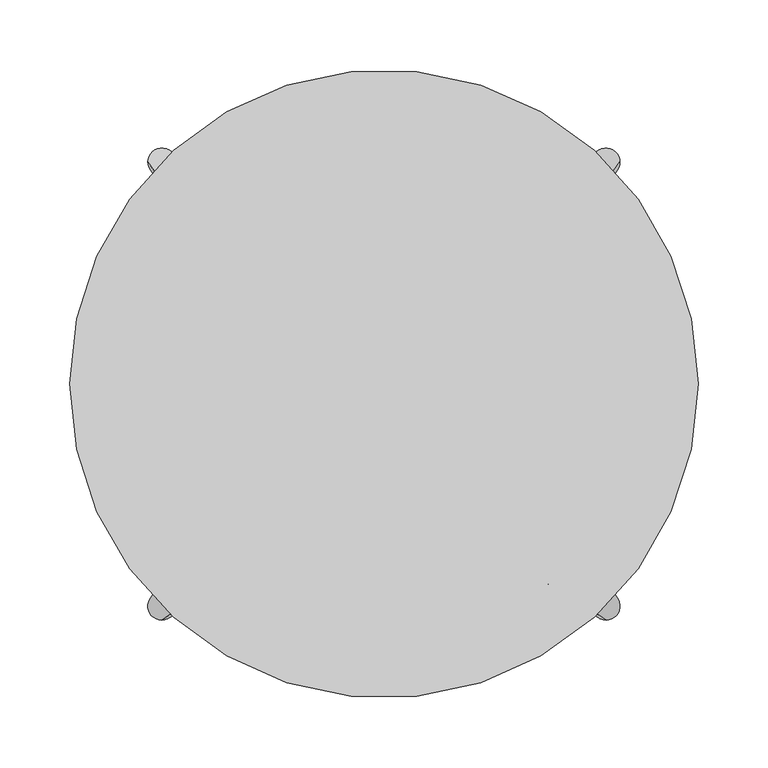
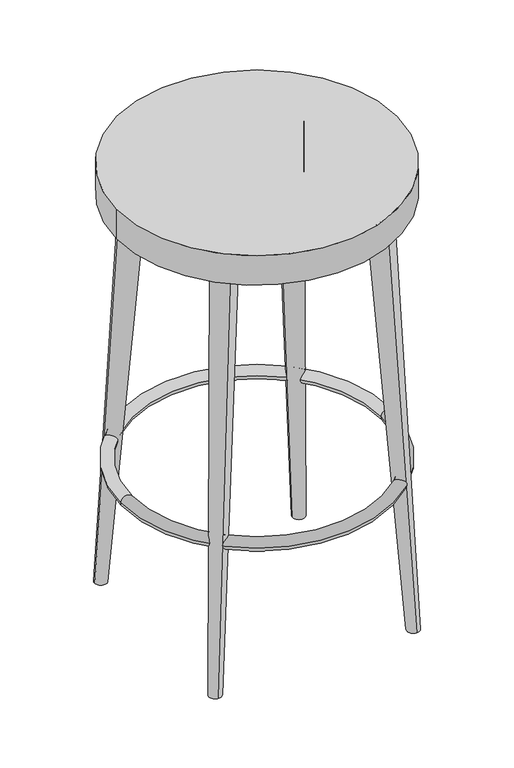
"""IFC4 building model written with IfcOpenShell, lengths in millimetres: furniture geometry."""

from ifc_helpers import new_model, si_unit, point, frame, origin, origin_2d, place, context, project, spatial, circle_curve, ellipse_curve, trimmed, segment, composite_curve, outline, extrude, source, transform, mapped, element, save
from ifc_brep_helpers import plane_surface, revolved_surface, spline_surface, advanced_brep


def furniture_d95c0d1d(model_context):
    return source(origin(), model_context, "Body", "SolidModel", [
        extrude(outline(composite_curve([segment(trimmed(circle_curve(origin_2d(), 225.0), [point((-225.0, 0.0))], [point((225.0, 0.0))], False, "CARTESIAN"), True, "CONTINUOUS"), segment(trimmed(circle_curve(origin_2d(), 225.0), [point((225.0, 0.0))], [point((-225.0, 0.0))], False, "CARTESIAN"), True, "CONTINUOUS")], self_intersect=False)), frame((0.0, 0.0, 700.0), z_axis=(0.0, 0.0, 1.0), x_axis=(1.0, 0.0, 0.0)), (0.0, 0.0, 1.0), 50.0),
        advanced_brep(
        [(-145.0, 125.0, 700.0), (-105.0, 125.0, 700.0), (-169.0990258, 159.0990258, 0.0), (-149.0990258, 159.0990258, 0.0)],
        [
            (0, 1, circle_curve(frame((-125.0, 125.0, 700.0), z_axis=(0.0, 0.0, 1.0), x_axis=(1.0, 0.0, 0.0)), 20.0)),
            (1, 0, circle_curve(frame((-125.0, 125.0, 700.0), z_axis=(0.0, 0.0, 1.0), x_axis=(1.0, 0.0, 0.0)), 20.0)),
            (2, 3, circle_curve(frame((-159.0990258, 159.0990258, 0.0), z_axis=(0.0, 0.0, -1.0), x_axis=(1.0, 0.0, 0.0)), 10.0)),
            (3, 2, circle_curve(frame((-159.0990258, 159.0990258, 0.0), z_axis=(0.0, 0.0, -1.0), x_axis=(1.0, 0.0, 0.0)), 10.0)),
            (3, 1),
            (0, 2),
        ],
        [
            plane_surface(frame((-125.0, 125.0, 700.0), z_axis=(0.0, 0.0, 1.0), x_axis=(0.0, -1.0, 0.0))),
            plane_surface(frame((-159.0990258, 159.0990258, 0.0), z_axis=(0.0, 0.0, -1.0), x_axis=(0.0, -1.0, 0.0))),
            spline_surface(2, 1, [[(-169.0990258, 159.0990258, 0.0), (-145.0, 125.0, 700.0)], [(-169.0990258, 149.0990258, 0.0), (-145.0, 105.0, 700.0)], [(-159.0990258, 149.0990258, 0.0), (-125.0, 105.0, 700.0)], [(-149.0990258, 149.0990258, 0.0), (-105.0, 105.0, 700.0)], [(-149.0990258, 159.0990258, 0.0), (-105.0, 125.0, 700.0)]], [3, 2, 3], [2, 2], [0.0, 1.0, 2.0], [0.0, 1.0], weights=[[1.0, 1.0], [0.7071067811865476, 0.7071067811865476], [1.0, 1.0], [0.7071067811865476, 0.7071067811865476], [1.0, 1.0]]),
            spline_surface(2, 1, [[(-149.0990258, 159.0990258, 0.0), (-105.0, 125.0, 700.0)], [(-149.0990258, 169.0990258, 0.0), (-105.0, 145.0, 700.0)], [(-159.0990258, 169.0990258, 0.0), (-125.0, 145.0, 700.0)], [(-169.0990258, 169.0990258, 0.0), (-145.0, 145.0, 700.0)], [(-169.0990258, 159.0990258, 0.0), (-145.0, 125.0, 700.0)]], [3, 2, 3], [2, 2], [0.0, 1.0, 2.0], [0.0, 1.0], weights=[[1.0, 1.0], [0.7071067811865476, 0.7071067811865476], [1.0, 1.0], [0.7071067811865476, 0.7071067811865476], [1.0, 1.0]]),
        ],
        [
            (0, [[1, 2]]),
            (1, [[3, 4]]),
            (2, [[-4, 5, -1, 6]]),
            (3, [[-3, -6, -2, -5]]),
        ],
    ),
        advanced_brep(
        [(125.0, -145.0, 700.0), (125.0, -105.0, 700.0), (159.0990258, -169.0990258, 0.0), (159.0990258, -149.0990258, 0.0)],
        [
            (0, 1, circle_curve(frame((125.0, -125.0, 700.0), z_axis=(0.0, 0.0, 1.0), x_axis=(0.0, 1.0, 0.0)), 20.0)),
            (1, 0, circle_curve(frame((125.0, -125.0, 700.0), z_axis=(0.0, 0.0, 1.0), x_axis=(0.0, 1.0, 0.0)), 20.0)),
            (2, 3, circle_curve(frame((159.0990258, -159.0990258, 0.0), z_axis=(0.0, 0.0, -1.0), x_axis=(0.0, 1.0, 0.0)), 10.0)),
            (3, 2, circle_curve(frame((159.0990258, -159.0990258, 0.0), z_axis=(0.0, 0.0, -1.0), x_axis=(0.0, 1.0, 0.0)), 10.0)),
            (2, 0),
            (1, 3),
        ],
        [
            plane_surface(frame((125.0, -125.0, 700.0), z_axis=(0.0, 0.0, 1.0), x_axis=(1.0, 0.0, 0.0))),
            plane_surface(frame((159.0990258, -159.0990258, 0.0), z_axis=(0.0, 0.0, -1.0), x_axis=(1.0, 0.0, 0.0))),
            spline_surface(2, 1, [[(159.0990258, -149.0990258, 0.0), (125.0, -105.0, 700.0)], [(149.0990258, -149.0990258, 0.0), (105.0, -105.0, 700.0)], [(149.0990258, -159.0990258, 0.0), (105.0, -125.0, 700.0)], [(149.0990258, -169.0990258, 0.0), (105.0, -145.0, 700.0)], [(159.0990258, -169.0990258, 0.0), (125.0, -145.0, 700.0)]], [3, 2, 3], [2, 2], [0.0, 1.0, 2.0], [0.0, 1.0], weights=[[1.0, 1.0], [0.7071067811865476, 0.7071067811865476], [1.0, 1.0], [0.7071067811865476, 0.7071067811865476], [1.0, 1.0]]),
            spline_surface(2, 1, [[(159.0990258, -169.0990258, 0.0), (125.0, -145.0, 700.0)], [(169.0990258, -169.0990258, 0.0), (145.0, -145.0, 700.0)], [(169.0990258, -159.0990258, 0.0), (145.0, -125.0, 700.0)], [(169.0990258, -149.0990258, 0.0), (145.0, -105.0, 700.0)], [(159.0990258, -149.0990258, 0.0), (125.0, -105.0, 700.0)]], [3, 2, 3], [2, 2], [0.0, 1.0, 2.0], [0.0, 1.0], weights=[[1.0, 1.0], [0.7071067811865476, 0.7071067811865476], [1.0, 1.0], [0.7071067811865476, 0.7071067811865476], [1.0, 1.0]]),
        ],
        [
            (0, [[1, 2]]),
            (1, [[3, 4]]),
            (2, [[-3, 5, -2, 6]]),
            (3, [[-4, -6, -1, -5]]),
        ],
    ),
        advanced_brep(
        [(145.0, 125.0, 700.0), (105.0, 125.0, 700.0), (169.0990258, 159.0990258, 0.0), (149.0990258, 159.0990258, 0.0)],
        [
            (0, 1, circle_curve(frame((125.0, 125.0, 700.0), z_axis=(0.0, 0.0, 1.0), x_axis=(-1.0, 0.0, 0.0)), 20.0)),
            (1, 0, circle_curve(frame((125.0, 125.0, 700.0), z_axis=(0.0, 0.0, 1.0), x_axis=(-1.0, 0.0, 0.0)), 20.0)),
            (2, 3, circle_curve(frame((159.0990258, 159.0990258, 0.0), z_axis=(0.0, 0.0, -1.0), x_axis=(-1.0, 0.0, 0.0)), 10.0)),
            (3, 2, circle_curve(frame((159.0990258, 159.0990258, 0.0), z_axis=(0.0, 0.0, -1.0), x_axis=(-1.0, 0.0, 0.0)), 10.0)),
            (2, 0),
            (1, 3),
        ],
        [
            plane_surface(frame((125.0, 125.0, 700.0), z_axis=(0.0, 0.0, 1.0), x_axis=(0.0, 1.0, 0.0))),
            plane_surface(frame((159.0990258, 159.0990258, 0.0), z_axis=(0.0, 0.0, -1.0), x_axis=(0.0, 1.0, 0.0))),
            spline_surface(2, 1, [[(149.0990258, 159.0990258, 0.0), (105.0, 125.0, 700.0)], [(149.0990258, 149.0990258, 0.0), (105.0, 105.0, 700.0)], [(159.0990258, 149.0990258, 0.0), (125.0, 105.0, 700.0)], [(169.0990258, 149.0990258, 0.0), (145.0, 105.0, 700.0)], [(169.0990258, 159.0990258, 0.0), (145.0, 125.0, 700.0)]], [3, 2, 3], [2, 2], [0.0, 1.0, 2.0], [0.0, 1.0], weights=[[1.0, 1.0], [0.7071067811865476, 0.7071067811865476], [1.0, 1.0], [0.7071067811865476, 0.7071067811865476], [1.0, 1.0]]),
            spline_surface(2, 1, [[(169.0990258, 159.0990258, 0.0), (145.0, 125.0, 700.0)], [(169.0990258, 169.0990258, 0.0), (145.0, 145.0, 700.0)], [(159.0990258, 169.0990258, 0.0), (125.0, 145.0, 700.0)], [(149.0990258, 169.0990258, 0.0), (105.0, 145.0, 700.0)], [(149.0990258, 159.0990258, 0.0), (105.0, 125.0, 700.0)]], [3, 2, 3], [2, 2], [0.0, 1.0, 2.0], [0.0, 1.0], weights=[[1.0, 1.0], [0.7071067811865476, 0.7071067811865476], [1.0, 1.0], [0.7071067811865476, 0.7071067811865476], [1.0, 1.0]]),
        ],
        [
            (0, [[1, 2]]),
            (1, [[3, 4]]),
            (2, [[-3, 5, -2, 6]]),
            (3, [[-4, -6, -1, -5]]),
        ],
    ),
        advanced_brep(
        [(-125.0, -145.0, 700.0), (-125.0, -105.0, 700.0), (-159.0990258, -169.0990258, 0.0), (-159.0990258, -149.0990258, 0.0)],
        [
            (0, 1, circle_curve(frame((-125.0, -125.0, 700.0), z_axis=(0.0, 0.0, 1.0), x_axis=(0.0, 1.0, 0.0)), 20.0)),
            (1, 0, circle_curve(frame((-125.0, -125.0, 700.0), z_axis=(0.0, 0.0, 1.0), x_axis=(0.0, 1.0, 0.0)), 20.0)),
            (2, 3, circle_curve(frame((-159.0990258, -159.0990258, 0.0), z_axis=(0.0, 0.0, -1.0), x_axis=(0.0, 1.0, 0.0)), 10.0)),
            (3, 2, circle_curve(frame((-159.0990258, -159.0990258, 0.0), z_axis=(0.0, 0.0, -1.0), x_axis=(0.0, 1.0, 0.0)), 10.0)),
            (3, 1),
            (0, 2),
        ],
        [
            plane_surface(frame((-125.0, -125.0, 700.0), z_axis=(0.0, 0.0, 1.0), x_axis=(1.0, 0.0, 0.0))),
            plane_surface(frame((-159.0990258, -159.0990258, 0.0), z_axis=(0.0, 0.0, -1.0), x_axis=(1.0, 0.0, 0.0))),
            spline_surface(2, 1, [[(-159.0990258, -169.0990258, 0.0), (-125.0, -145.0, 700.0)], [(-149.0990258, -169.0990258, 0.0), (-105.0, -145.0, 700.0)], [(-149.0990258, -159.0990258, 0.0), (-105.0, -125.0, 700.0)], [(-149.0990258, -149.0990258, 0.0), (-105.0, -105.0, 700.0)], [(-159.0990258, -149.0990258, 0.0), (-125.0, -105.0, 700.0)]], [3, 2, 3], [2, 2], [0.0, 1.0, 2.0], [0.0, 1.0], weights=[[1.0, 1.0], [0.7071067811865476, 0.7071067811865476], [1.0, 1.0], [0.7071067811865476, 0.7071067811865476], [1.0, 1.0]]),
            spline_surface(2, 1, [[(-159.0990258, -149.0990258, 0.0), (-125.0, -105.0, 700.0)], [(-169.0990258, -149.0990258, 0.0), (-145.0, -105.0, 700.0)], [(-169.0990258, -159.0990258, 0.0), (-145.0, -125.0, 700.0)], [(-169.0990258, -169.0990258, 0.0), (-145.0, -145.0, 700.0)], [(-159.0990258, -169.0990258, 0.0), (-125.0, -145.0, 700.0)]], [3, 2, 3], [2, 2], [0.0, 1.0, 2.0], [0.0, 1.0], weights=[[1.0, 1.0], [0.7071067811865476, 0.7071067811865476], [1.0, 1.0], [0.7071067811865476, 0.7071067811865476], [1.0, 1.0]]),
        ],
        [
            (0, [[1, 2]]),
            (1, [[3, 4]]),
            (2, [[-4, 5, -1, 6]]),
            (3, [[-3, -6, -2, -5]]),
        ],
    ),
        advanced_brep(
        [(198.8927572, 0.0, 250.0), (-198.8927572, 0.0, 250.0), (-218.8927572, 0.0, 250.0), (218.8927572, 0.0, 250.0)],
        [
            (0, 1, circle_curve(frame((0.0, 0.0, 250.0), z_axis=(0.0, 0.0, 1.0), x_axis=(-1.0, 0.0, 0.0)), 198.8927572)),
            (1, 2, circle_curve(frame((-208.8927572, 0.0, 250.0), z_axis=(0.0, 1.0, 0.0), x_axis=(1.0, 0.0, 0.0)), 10.0)),
            (2, 3, circle_curve(frame((0.0, 0.0, 250.0), z_axis=(0.0, 0.0, -1.0), x_axis=(-1.0, 0.0, 0.0)), 218.8927572)),
            (3, 0, circle_curve(frame((208.8927572, 0.0, 250.0), z_axis=(0.0, 1.0, 0.0), x_axis=(-1.0, 0.0, 0.0)), 10.0)),
            (1, 0, circle_curve(frame((0.0, 0.0, 250.0), z_axis=(0.0, 0.0, 1.0), x_axis=(-1.0, 0.0, 0.0)), 198.8927572)),
            (3, 2, circle_curve(frame((0.0, 0.0, 250.0), z_axis=(0.0, 0.0, -1.0), x_axis=(-1.0, 0.0, 0.0)), 218.8927572)),
            (2, 1, circle_curve(frame((-208.8927572, 0.0, 250.0), z_axis=(0.0, 1.0, 0.0), x_axis=(1.0, 0.0, 0.0)), 10.0)),
            (0, 3, circle_curve(frame((208.8927572, 0.0, 250.0), z_axis=(0.0, 1.0, 0.0), x_axis=(-1.0, 0.0, 0.0)), 10.0)),
        ],
        [
            revolved_surface(trimmed(ellipse_curve(frame((-208.8927572, 0.0, 250.0), z_axis=(0.0, -1.0, 0.0), x_axis=(1.0, 0.0, 0.0)), 10.0, 10.0), [point((-218.8927572, 0.0, 250.0))], [point((-198.8927572, 0.0, 250.0))], True, "CARTESIAN"), (0.0, 0.0, 580.0), (0.0, 0.0, -1.0)),
            revolved_surface(trimmed(ellipse_curve(frame((-208.8927572, 0.0, 250.0), z_axis=(0.0, -1.0, 0.0), x_axis=(1.0, 0.0, 0.0)), 10.0, 10.0), [point((-198.8927572, 0.0, 250.0))], [point((-218.8927572, 0.0, 250.0))], True, "CARTESIAN"), (0.0, 0.0, 580.0), (0.0, 0.0, -1.0)),
        ],
        [
            (0, [[1, 2, 3, 4]]),
            (0, [[5, -4, 6, -2]]),
            (1, [[-3, 7, -1, 8]]),
            (1, [[-6, -8, -5, -7]]),
        ],
    ),
    ])


if __name__ == "__main__":
    model = new_model("IFC4")
    model_context = context("Model", 3, world=origin())
    ifc_project = project(units=[si_unit("LENGTHUNIT", "METRE", prefix="MILLI")], contexts=[model_context])
    site = spatial("IfcSite", under=ifc_project)
    building = spatial("IfcBuilding", under=site)
    placement = place(None, origin())
    furniture_shape = furniture_d95c0d1d(model_context)
    element("IfcFurniture", 1, at=placement, inside=building, context=model_context, shape_type="MappedRepresentation", body=[
        mapped(furniture_shape, transform((0.0, 0.0, 0.0), x_axis=(1.0, 0.0, 0.0), y_axis=(0.0, 1.0, 0.0), z_axis=(0.0, 0.0, 1.0))),
    ])
    save(model, "model.ifc")

# Revit data of these elements
# Type
#   Default Elevation = 0
# Element 1 (IfcFurniture)
#   Materials on its faces: "Metal - Chrome", "Wood - Birch"
# Materials
#   "Metal - Chrome": colour RGB 177 177 177, transparency 0
#   "Wood - Birch": colour RGB 210 159 95, transparency 0
